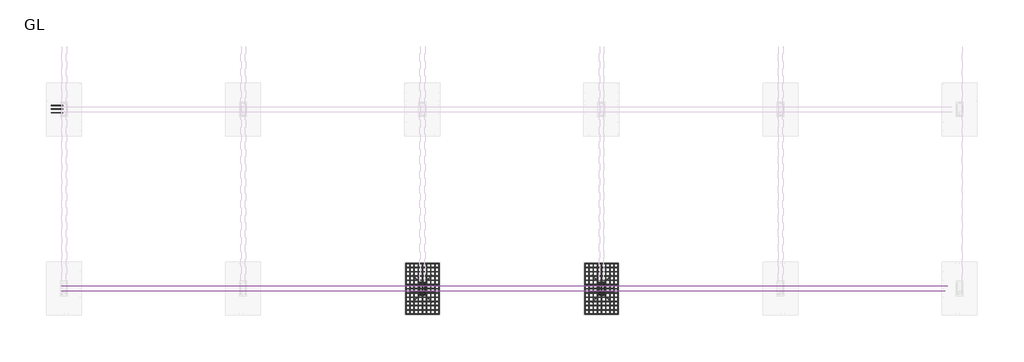
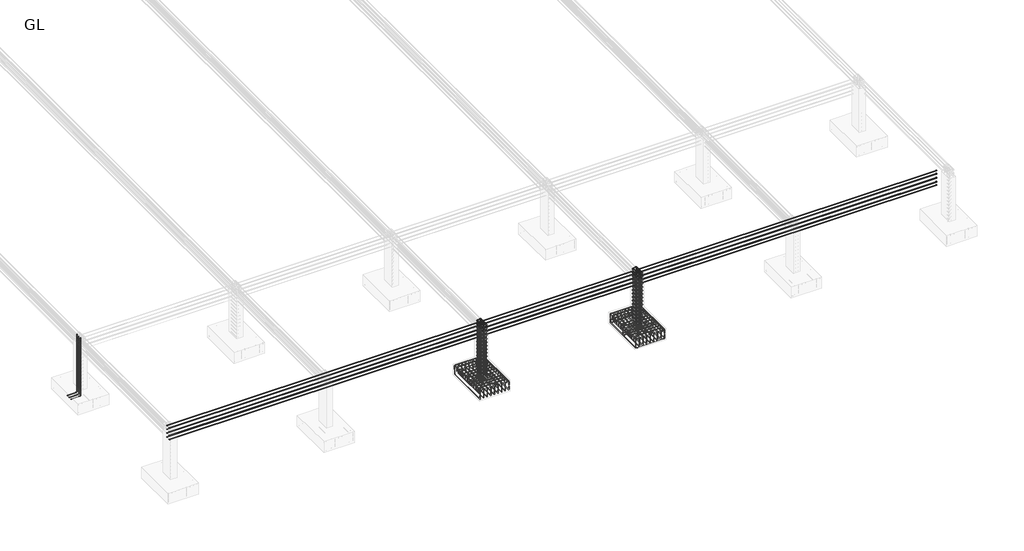
# One storey, part 3 of 16: 24 reinforcing bars.
"""IFC4 building model written with IfcOpenShell, lengths in millimetres."""

from ifc_helpers import new_model, si_unit, point, frame, origin, place, context, project, spatial, polyline, circle_curve, trimmed, segment, composite_curve, source, transform, mapped, element, save
from ifc_brep_helpers import swept_disk

model = new_model("IFC4")

# Units and contexts
model_context = context("Model", 3, world=origin())
ifc_project = project(units=[si_unit("LENGTHUNIT", "METRE", prefix="MILLI")], contexts=[model_context])

# Site, building, storey
site = spatial("IfcSite", under=ifc_project)
building = spatial("IfcBuilding", under=site)
storey = spatial("IfcBuildingStorey", under=building, Name="GL", Elevation=-1829.0)

# Reinforcing bars
placement = place(None, origin())
reinforcing_bar_shape = source(origin(), model_context, "Body", "SolidModel", [
    swept_disk(composite_curve([segment(polyline([(-11178.9544379, -19415.1167521, -2022.436678), (-11178.9544379, -19415.1167521, -1898.436678)]), True, "CONTINUOUS"), segment(trimmed(circle_curve(frame((-11148.9544379, -19415.1167521, -1898.436678), z_axis=(0.0, 1.0, 0.0), x_axis=(-30.0, 0.0, 0.0)), 30.0), [point((-11178.9544379, -19415.1167521, -1898.436678))], [point((-11148.9544379, -19415.1167521, -1868.436678))], True, "CARTESIAN"), True, "CONTINUOUS"), segment(polyline([(-11148.9544379, -19415.1167521, -1868.436678), (-10080.9544379, -19415.1167521, -1868.436678)]), True, "CONTINUOUS"), segment(trimmed(circle_curve(frame((-10080.9544379, -19415.1167521, -1898.436678), z_axis=(0.0, 1.0, 0.0), x_axis=(0.0, 0.0, 30.0)), 30.0), [point((-10080.9544379, -19415.1167521, -1868.436678))], [point((-10050.9544379, -19415.1167521, -1898.436678))], True, "CARTESIAN"), True, "CONTINUOUS"), segment(polyline([(-10050.9544379, -19415.1167521, -1898.436678), (-10050.9544379, -19415.1167521, -2022.436678)]), True, "CONTINUOUS")], self_intersect=False), 6.0),
])
element("IfcReinforcingBar", 1, at=placement, inside=storey, context=model_context, shape_type="MappedRepresentation", body=[
    mapped(reinforcing_bar_shape, transform((0.0, 0.0, 0.0), x_axis=(1.0, 0.0, 0.0), y_axis=(0.0, 1.0, 0.0), z_axis=(0.0, 0.0, 1.0))),
    mapped(reinforcing_bar_shape, transform((0.0, -144.0, 0.0), x_axis=(1.0, 0.0, 0.0), y_axis=(0.0, 1.0, 0.0), z_axis=(0.0, 0.0, 1.0))),
    mapped(reinforcing_bar_shape, transform((0.0, -288.0, 0.0), x_axis=(1.0, 0.0, 0.0), y_axis=(0.0, 1.0, 0.0), z_axis=(0.0, 0.0, 1.0))),
    mapped(reinforcing_bar_shape, transform((0.0, -432.0, 0.0), x_axis=(1.0, 0.0, 0.0), y_axis=(0.0, 1.0, 0.0), z_axis=(0.0, 0.0, 1.0))),
    mapped(reinforcing_bar_shape, transform((0.0, -576.0, 0.0), x_axis=(1.0, 0.0, 0.0), y_axis=(0.0, 1.0, 0.0), z_axis=(0.0, 0.0, 1.0))),
    mapped(reinforcing_bar_shape, transform((0.0, -720.0, 0.0), x_axis=(1.0, 0.0, 0.0), y_axis=(0.0, 1.0, 0.0), z_axis=(0.0, 0.0, 1.0))),
    mapped(reinforcing_bar_shape, transform((0.0, -864.0, 0.0), x_axis=(1.0, 0.0, 0.0), y_axis=(0.0, 1.0, 0.0), z_axis=(0.0, 0.0, 1.0))),
    mapped(reinforcing_bar_shape, transform((0.0, -1008.0, 0.0), x_axis=(1.0, 0.0, 0.0), y_axis=(0.0, 1.0, 0.0), z_axis=(0.0, 0.0, 1.0))),
    mapped(reinforcing_bar_shape, transform((0.0, -1152.0, 0.0), x_axis=(1.0, 0.0, 0.0), y_axis=(0.0, 1.0, 0.0), z_axis=(0.0, 0.0, 1.0))),
    mapped(reinforcing_bar_shape, transform((0.0, -1296.0, 0.0), x_axis=(1.0, 0.0, 0.0), y_axis=(0.0, 1.0, 0.0), z_axis=(0.0, 0.0, 1.0))),
    mapped(reinforcing_bar_shape, transform((0.0, -1440.0, 0.0), x_axis=(1.0, 0.0, 0.0), y_axis=(0.0, 1.0, 0.0), z_axis=(0.0, 0.0, 1.0))),
    mapped(reinforcing_bar_shape, transform((0.0, -1584.0, 0.0), x_axis=(1.0, 0.0, 0.0), y_axis=(0.0, 1.0, 0.0), z_axis=(0.0, 0.0, 1.0))),
    mapped(reinforcing_bar_shape, transform((0.0, -1728.0, 0.0), x_axis=(1.0, 0.0, 0.0), y_axis=(0.0, 1.0, 0.0), z_axis=(0.0, 0.0, 1.0))),
])
reinforcing_bar_2_shape = source(origin(), model_context, "Body", "SolidModel", [
    swept_disk(composite_curve([segment(polyline([(-11178.9544379, -21143.1167521, -2027.5081232), (-11178.9544379, -21143.1167521, -1903.5081232)]), True, "CONTINUOUS"), segment(trimmed(circle_curve(frame((-11178.9544379, -21113.1167521, -1903.5081232), z_axis=(-1.0, 0.0, 0.0), x_axis=(0.0, -30.0, 0.0)), 30.0), [point((-11178.9544379, -21143.1167521, -1903.5081232))], [point((-11178.9544379, -21113.1167521, -1873.5081232))], True, "CARTESIAN"), True, "CONTINUOUS"), segment(polyline([(-11178.9544379, -21113.1167521, -1873.5081232), (-11178.9544379, -19445.1167521, -1873.5081232)]), True, "CONTINUOUS"), segment(trimmed(circle_curve(frame((-11178.9544379, -19445.1167521, -1903.5081232), z_axis=(-1.0, 0.0, 0.0), x_axis=(0.0, 0.0, 30.0)), 30.0), [point((-11178.9544379, -19445.1167521, -1873.5081232))], [point((-11178.9544379, -19415.1167521, -1903.5081232))], True, "CARTESIAN"), True, "CONTINUOUS"), segment(polyline([(-11178.9544379, -19415.1167521, -1903.5081232), (-11178.9544379, -19415.1167521, -2027.5081232)]), True, "CONTINUOUS")], self_intersect=False), 6.0),
])
element("IfcReinforcingBar", 2, at=placement, inside=storey, context=model_context, shape_type="MappedRepresentation", body=[
    mapped(reinforcing_bar_2_shape, transform((0.0, 0.0, 0.0), x_axis=(1.0, 0.0, 0.0), y_axis=(0.0, 1.0, 0.0), z_axis=(0.0, 0.0, 1.0))),
    mapped(reinforcing_bar_2_shape, transform((141.0, 0.0, 0.0), x_axis=(1.0, 0.0, 0.0), y_axis=(0.0, 1.0, 0.0), z_axis=(0.0, 0.0, 1.0))),
    mapped(reinforcing_bar_2_shape, transform((282.0, 0.0, 0.0), x_axis=(1.0, 0.0, 0.0), y_axis=(0.0, 1.0, 0.0), z_axis=(0.0, 0.0, 1.0))),
    mapped(reinforcing_bar_2_shape, transform((423.0, 0.0, 0.0), x_axis=(1.0, 0.0, 0.0), y_axis=(0.0, 1.0, 0.0), z_axis=(0.0, 0.0, 1.0))),
    mapped(reinforcing_bar_2_shape, transform((564.0, 0.0, 0.0), x_axis=(1.0, 0.0, 0.0), y_axis=(0.0, 1.0, 0.0), z_axis=(0.0, 0.0, 1.0))),
    mapped(reinforcing_bar_2_shape, transform((705.0, 0.0, 0.0), x_axis=(1.0, 0.0, 0.0), y_axis=(0.0, 1.0, 0.0), z_axis=(0.0, 0.0, 1.0))),
    mapped(reinforcing_bar_2_shape, transform((846.0, 0.0, 0.0), x_axis=(1.0, 0.0, 0.0), y_axis=(0.0, 1.0, 0.0), z_axis=(0.0, 0.0, 1.0))),
    mapped(reinforcing_bar_2_shape, transform((987.0, 0.0, 0.0), x_axis=(1.0, 0.0, 0.0), y_axis=(0.0, 1.0, 0.0), z_axis=(0.0, 0.0, 1.0))),
    mapped(reinforcing_bar_2_shape, transform((1128.0, 0.0, 0.0), x_axis=(1.0, 0.0, 0.0), y_axis=(0.0, 1.0, 0.0), z_axis=(0.0, 0.0, 1.0))),
])
reinforcing_bar_3_shape = source(origin(), model_context, "Body", "SolidModel", [
    swept_disk(composite_curve([segment(polyline([(-10050.9544379, -21143.1167521, -2080.6239909), (-10050.9544379, -21143.1167521, -2204.6239909)]), True, "CONTINUOUS"), segment(trimmed(circle_curve(frame((-10050.9544379, -21113.1167521, -2204.6239909), z_axis=(1.0, 0.0, 0.0), x_axis=(0.0, -30.0, 0.0)), 30.0), [point((-10050.9544379, -21143.1167521, -2204.6239909))], [point((-10050.9544379, -21113.1167521, -2234.6239909))], True, "CARTESIAN"), True, "CONTINUOUS"), segment(polyline([(-10050.9544379, -21113.1167521, -2234.6239909), (-10050.9544379, -19458.1421892, -2234.6239909)]), True, "CONTINUOUS"), segment(trimmed(circle_curve(frame((-10050.9544379, -19458.1421892, -2204.6239909), z_axis=(1.0, 0.0, 0.0), x_axis=(0.0, 0.0, -30.0)), 30.0), [point((-10050.9544379, -19458.1421892, -2234.6239909))], [point((-10050.9544379, -19428.1421892, -2204.6239909))], True, "CARTESIAN"), True, "CONTINUOUS"), segment(polyline([(-10050.9544379, -19428.1421892, -2204.6239909), (-10050.9544379, -19428.1421892, -2080.6239909)]), True, "CONTINUOUS")], self_intersect=False), 6.0),
])
element("IfcReinforcingBar", 3, at=placement, inside=storey, context=model_context, shape_type="MappedRepresentation", body=[
    mapped(reinforcing_bar_3_shape, transform((0.0, 0.0, 0.0), x_axis=(1.0, 0.0, 0.0), y_axis=(0.0, 1.0, 0.0), z_axis=(0.0, 0.0, 1.0))),
    mapped(reinforcing_bar_3_shape, transform((-141.0, 0.0, 0.0), x_axis=(1.0, 0.0, 0.0), y_axis=(0.0, 1.0, 0.0), z_axis=(0.0, 0.0, 1.0))),
    mapped(reinforcing_bar_3_shape, transform((-282.0, 0.0, 0.0), x_axis=(1.0, 0.0, 0.0), y_axis=(0.0, 1.0, 0.0), z_axis=(0.0, 0.0, 1.0))),
    mapped(reinforcing_bar_3_shape, transform((-423.0, 0.0, 0.0), x_axis=(1.0, 0.0, 0.0), y_axis=(0.0, 1.0, 0.0), z_axis=(0.0, 0.0, 1.0))),
    mapped(reinforcing_bar_3_shape, transform((-564.0, 0.0, 0.0), x_axis=(1.0, 0.0, 0.0), y_axis=(0.0, 1.0, 0.0), z_axis=(0.0, 0.0, 1.0))),
    mapped(reinforcing_bar_3_shape, transform((-705.0, 0.0, 0.0), x_axis=(1.0, 0.0, 0.0), y_axis=(0.0, 1.0, 0.0), z_axis=(0.0, 0.0, 1.0))),
    mapped(reinforcing_bar_3_shape, transform((-846.0, 0.0, 0.0), x_axis=(1.0, 0.0, 0.0), y_axis=(0.0, 1.0, 0.0), z_axis=(0.0, 0.0, 1.0))),
    mapped(reinforcing_bar_3_shape, transform((-987.0, 0.0, 0.0), x_axis=(1.0, 0.0, 0.0), y_axis=(0.0, 1.0, 0.0), z_axis=(0.0, 0.0, 1.0))),
    mapped(reinforcing_bar_3_shape, transform((-1128.0, 0.0, 0.0), x_axis=(1.0, 0.0, 0.0), y_axis=(0.0, 1.0, 0.0), z_axis=(0.0, 0.0, 1.0))),
])
reinforcing_bar_4_shape = source(origin(), model_context, "Body", "SolidModel", [
    swept_disk(composite_curve([segment(polyline([(-3954.9544379, -19415.1167521, -2089.0), (-3954.9544379, -19415.1167521, -2213.0)]), True, "CONTINUOUS"), segment(trimmed(circle_curve(frame((-3984.9544379, -19415.1167521, -2213.0), z_axis=(0.0, 1.0, 0.0), x_axis=(30.0, 0.0, 0.0)), 30.0), [point((-3954.9544379, -19415.1167521, -2213.0))], [point((-3984.9544379, -19415.1167521, -2243.0))], True, "CARTESIAN"), True, "CONTINUOUS"), segment(polyline([(-3984.9544379, -19415.1167521, -2243.0), (-5052.9544379, -19415.1167521, -2243.0)]), True, "CONTINUOUS"), segment(trimmed(circle_curve(frame((-5052.9544379, -19415.1167521, -2213.0), z_axis=(0.0, 1.0, 0.0), x_axis=(0.0, 0.0, -30.0)), 30.0), [point((-5052.9544379, -19415.1167521, -2243.0))], [point((-5082.9544379, -19415.1167521, -2213.0))], True, "CARTESIAN"), True, "CONTINUOUS"), segment(polyline([(-5082.9544379, -19415.1167521, -2213.0), (-5082.9544379, -19415.1167521, -2089.0)]), True, "CONTINUOUS")], self_intersect=False), 6.0),
])
element("IfcReinforcingBar", 4, at=placement, inside=storey, context=model_context, shape_type="MappedRepresentation", body=[
    mapped(reinforcing_bar_4_shape, transform((0.0, 0.0, 0.0), x_axis=(1.0, 0.0, 0.0), y_axis=(0.0, 1.0, 0.0), z_axis=(0.0, 0.0, 1.0))),
    mapped(reinforcing_bar_4_shape, transform((0.0, -864.0, 0.0), x_axis=(1.0, 0.0, 0.0), y_axis=(0.0, 1.0, 0.0), z_axis=(0.0, 0.0, 1.0))),
    mapped(reinforcing_bar_4_shape, transform((0.0, -1728.0, 0.0), x_axis=(1.0, 0.0, 0.0), y_axis=(0.0, 1.0, 0.0), z_axis=(0.0, 0.0, 1.0))),
])
reinforcing_bar_5_shape = source(origin(), model_context, "Body", "SolidModel", [
    swept_disk(composite_curve([segment(polyline([(-5082.9544379, -19415.1167521, -2022.436678), (-5082.9544379, -19415.1167521, -1898.436678)]), True, "CONTINUOUS"), segment(trimmed(circle_curve(frame((-5052.9544379, -19415.1167521, -1898.436678), z_axis=(0.0, 1.0, 0.0), x_axis=(-30.0, 0.0, 0.0)), 30.0), [point((-5082.9544379, -19415.1167521, -1898.436678))], [point((-5052.9544379, -19415.1167521, -1868.436678))], True, "CARTESIAN"), True, "CONTINUOUS"), segment(polyline([(-5052.9544379, -19415.1167521, -1868.436678), (-3984.9544379, -19415.1167521, -1868.436678)]), True, "CONTINUOUS"), segment(trimmed(circle_curve(frame((-3984.9544379, -19415.1167521, -1898.436678), z_axis=(0.0, 1.0, 0.0), x_axis=(0.0, 0.0, 30.0)), 30.0), [point((-3984.9544379, -19415.1167521, -1868.436678))], [point((-3954.9544379, -19415.1167521, -1898.436678))], True, "CARTESIAN"), True, "CONTINUOUS"), segment(polyline([(-3954.9544379, -19415.1167521, -1898.436678), (-3954.9544379, -19415.1167521, -2022.436678)]), True, "CONTINUOUS")], self_intersect=False), 6.0),
])
element("IfcReinforcingBar", 5, at=placement, inside=storey, context=model_context, shape_type="MappedRepresentation", body=[
    mapped(reinforcing_bar_5_shape, transform((0.0, 0.0, 0.0), x_axis=(1.0, 0.0, 0.0), y_axis=(0.0, 1.0, 0.0), z_axis=(0.0, 0.0, 1.0))),
    mapped(reinforcing_bar_5_shape, transform((0.0, -144.0, 0.0), x_axis=(1.0, 0.0, 0.0), y_axis=(0.0, 1.0, 0.0), z_axis=(0.0, 0.0, 1.0))),
    mapped(reinforcing_bar_5_shape, transform((0.0, -288.0, 0.0), x_axis=(1.0, 0.0, 0.0), y_axis=(0.0, 1.0, 0.0), z_axis=(0.0, 0.0, 1.0))),
    mapped(reinforcing_bar_5_shape, transform((0.0, -432.0, 0.0), x_axis=(1.0, 0.0, 0.0), y_axis=(0.0, 1.0, 0.0), z_axis=(0.0, 0.0, 1.0))),
    mapped(reinforcing_bar_5_shape, transform((0.0, -576.0, 0.0), x_axis=(1.0, 0.0, 0.0), y_axis=(0.0, 1.0, 0.0), z_axis=(0.0, 0.0, 1.0))),
    mapped(reinforcing_bar_5_shape, transform((0.0, -720.0, 0.0), x_axis=(1.0, 0.0, 0.0), y_axis=(0.0, 1.0, 0.0), z_axis=(0.0, 0.0, 1.0))),
    mapped(reinforcing_bar_5_shape, transform((0.0, -864.0, 0.0), x_axis=(1.0, 0.0, 0.0), y_axis=(0.0, 1.0, 0.0), z_axis=(0.0, 0.0, 1.0))),
    mapped(reinforcing_bar_5_shape, transform((0.0, -1008.0, 0.0), x_axis=(1.0, 0.0, 0.0), y_axis=(0.0, 1.0, 0.0), z_axis=(0.0, 0.0, 1.0))),
    mapped(reinforcing_bar_5_shape, transform((0.0, -1152.0, 0.0), x_axis=(1.0, 0.0, 0.0), y_axis=(0.0, 1.0, 0.0), z_axis=(0.0, 0.0, 1.0))),
    mapped(reinforcing_bar_5_shape, transform((0.0, -1296.0, 0.0), x_axis=(1.0, 0.0, 0.0), y_axis=(0.0, 1.0, 0.0), z_axis=(0.0, 0.0, 1.0))),
    mapped(reinforcing_bar_5_shape, transform((0.0, -1440.0, 0.0), x_axis=(1.0, 0.0, 0.0), y_axis=(0.0, 1.0, 0.0), z_axis=(0.0, 0.0, 1.0))),
    mapped(reinforcing_bar_5_shape, transform((0.0, -1584.0, 0.0), x_axis=(1.0, 0.0, 0.0), y_axis=(0.0, 1.0, 0.0), z_axis=(0.0, 0.0, 1.0))),
    mapped(reinforcing_bar_5_shape, transform((0.0, -1728.0, 0.0), x_axis=(1.0, 0.0, 0.0), y_axis=(0.0, 1.0, 0.0), z_axis=(0.0, 0.0, 1.0))),
])
reinforcing_bar_6_shape = source(origin(), model_context, "Body", "SolidModel", [
    swept_disk(composite_curve([segment(polyline([(-5082.9544379, -21143.1167521, -2027.5081232), (-5082.9544379, -21143.1167521, -1903.5081232)]), True, "CONTINUOUS"), segment(trimmed(circle_curve(frame((-5082.9544379, -21113.1167521, -1903.5081232), z_axis=(-1.0, 0.0, 0.0), x_axis=(0.0, -30.0, 0.0)), 30.0), [point((-5082.9544379, -21143.1167521, -1903.5081232))], [point((-5082.9544379, -21113.1167521, -1873.5081232))], True, "CARTESIAN"), True, "CONTINUOUS"), segment(polyline([(-5082.9544379, -21113.1167521, -1873.5081232), (-5082.9544379, -19445.1167521, -1873.5081232)]), True, "CONTINUOUS"), segment(trimmed(circle_curve(frame((-5082.9544379, -19445.1167521, -1903.5081232), z_axis=(-1.0, 0.0, 0.0), x_axis=(0.0, 0.0, 30.0)), 30.0), [point((-5082.9544379, -19445.1167521, -1873.5081232))], [point((-5082.9544379, -19415.1167521, -1903.5081232))], True, "CARTESIAN"), True, "CONTINUOUS"), segment(polyline([(-5082.9544379, -19415.1167521, -1903.5081232), (-5082.9544379, -19415.1167521, -2027.5081232)]), True, "CONTINUOUS")], self_intersect=False), 6.0),
])
element("IfcReinforcingBar", 6, at=placement, inside=storey, context=model_context, shape_type="MappedRepresentation", body=[
    mapped(reinforcing_bar_6_shape, transform((0.0, 0.0, 0.0), x_axis=(1.0, 0.0, 0.0), y_axis=(0.0, 1.0, 0.0), z_axis=(0.0, 0.0, 1.0))),
    mapped(reinforcing_bar_6_shape, transform((141.0, 0.0, 0.0), x_axis=(1.0, 0.0, 0.0), y_axis=(0.0, 1.0, 0.0), z_axis=(0.0, 0.0, 1.0))),
    mapped(reinforcing_bar_6_shape, transform((282.0, 0.0, 0.0), x_axis=(1.0, 0.0, 0.0), y_axis=(0.0, 1.0, 0.0), z_axis=(0.0, 0.0, 1.0))),
    mapped(reinforcing_bar_6_shape, transform((423.0, 0.0, 0.0), x_axis=(1.0, 0.0, 0.0), y_axis=(0.0, 1.0, 0.0), z_axis=(0.0, 0.0, 1.0))),
    mapped(reinforcing_bar_6_shape, transform((564.0, 0.0, 0.0), x_axis=(1.0, 0.0, 0.0), y_axis=(0.0, 1.0, 0.0), z_axis=(0.0, 0.0, 1.0))),
    mapped(reinforcing_bar_6_shape, transform((705.0, 0.0, 0.0), x_axis=(1.0, 0.0, 0.0), y_axis=(0.0, 1.0, 0.0), z_axis=(0.0, 0.0, 1.0))),
    mapped(reinforcing_bar_6_shape, transform((846.0, 0.0, 0.0), x_axis=(1.0, 0.0, 0.0), y_axis=(0.0, 1.0, 0.0), z_axis=(0.0, 0.0, 1.0))),
    mapped(reinforcing_bar_6_shape, transform((987.0, 0.0, 0.0), x_axis=(1.0, 0.0, 0.0), y_axis=(0.0, 1.0, 0.0), z_axis=(0.0, 0.0, 1.0))),
    mapped(reinforcing_bar_6_shape, transform((1128.0, 0.0, 0.0), x_axis=(1.0, 0.0, 0.0), y_axis=(0.0, 1.0, 0.0), z_axis=(0.0, 0.0, 1.0))),
])
reinforcing_bar_7_shape = source(origin(), model_context, "Body", "SolidModel", [
    swept_disk(composite_curve([segment(polyline([(-3954.9544379, -21143.1167521, -2080.6239909), (-3954.9544379, -21143.1167521, -2204.6239909)]), True, "CONTINUOUS"), segment(trimmed(circle_curve(frame((-3954.9544379, -21113.1167521, -2204.6239909), z_axis=(1.0, 0.0, 0.0), x_axis=(0.0, -30.0, 0.0)), 30.0), [point((-3954.9544379, -21143.1167521, -2204.6239909))], [point((-3954.9544379, -21113.1167521, -2234.6239909))], True, "CARTESIAN"), True, "CONTINUOUS"), segment(polyline([(-3954.9544379, -21113.1167521, -2234.6239909), (-3954.9544379, -19458.1421892, -2234.6239909)]), True, "CONTINUOUS"), segment(trimmed(circle_curve(frame((-3954.9544379, -19458.1421892, -2204.6239909), z_axis=(1.0, 0.0, 0.0), x_axis=(0.0, 0.0, -30.0)), 30.0), [point((-3954.9544379, -19458.1421892, -2234.6239909))], [point((-3954.9544379, -19428.1421892, -2204.6239909))], True, "CARTESIAN"), True, "CONTINUOUS"), segment(polyline([(-3954.9544379, -19428.1421892, -2204.6239909), (-3954.9544379, -19428.1421892, -2080.6239909)]), True, "CONTINUOUS")], self_intersect=False), 6.0),
])
element("IfcReinforcingBar", 7, at=placement, inside=storey, context=model_context, shape_type="MappedRepresentation", body=[
    mapped(reinforcing_bar_7_shape, transform((0.0, 0.0, 0.0), x_axis=(1.0, 0.0, 0.0), y_axis=(0.0, 1.0, 0.0), z_axis=(0.0, 0.0, 1.0))),
    mapped(reinforcing_bar_7_shape, transform((-141.0, 0.0, 0.0), x_axis=(1.0, 0.0, 0.0), y_axis=(0.0, 1.0, 0.0), z_axis=(0.0, 0.0, 1.0))),
    mapped(reinforcing_bar_7_shape, transform((-282.0, 0.0, 0.0), x_axis=(1.0, 0.0, 0.0), y_axis=(0.0, 1.0, 0.0), z_axis=(0.0, 0.0, 1.0))),
    mapped(reinforcing_bar_7_shape, transform((-423.0, 0.0, 0.0), x_axis=(1.0, 0.0, 0.0), y_axis=(0.0, 1.0, 0.0), z_axis=(0.0, 0.0, 1.0))),
    mapped(reinforcing_bar_7_shape, transform((-564.0, 0.0, 0.0), x_axis=(1.0, 0.0, 0.0), y_axis=(0.0, 1.0, 0.0), z_axis=(0.0, 0.0, 1.0))),
    mapped(reinforcing_bar_7_shape, transform((-705.0, 0.0, 0.0), x_axis=(1.0, 0.0, 0.0), y_axis=(0.0, 1.0, 0.0), z_axis=(0.0, 0.0, 1.0))),
    mapped(reinforcing_bar_7_shape, transform((-846.0, 0.0, 0.0), x_axis=(1.0, 0.0, 0.0), y_axis=(0.0, 1.0, 0.0), z_axis=(0.0, 0.0, 1.0))),
    mapped(reinforcing_bar_7_shape, transform((-987.0, 0.0, 0.0), x_axis=(1.0, 0.0, 0.0), y_axis=(0.0, 1.0, 0.0), z_axis=(0.0, 0.0, 1.0))),
    mapped(reinforcing_bar_7_shape, transform((-1128.0, 0.0, 0.0), x_axis=(1.0, 0.0, 0.0), y_axis=(0.0, 1.0, 0.0), z_axis=(0.0, 0.0, 1.0))),
])
reinforcing_bar_8_shape = source(origin(), model_context, "Body", "SolidModel", [
    swept_disk(composite_curve([segment(polyline([(-22864.0642232, -14290.9117405, 241.0), (-22864.0642232, -14290.9117405, -2129.0)]), True, "CONTINUOUS"), segment(trimmed(circle_curve(frame((-22894.0642232, -14290.9117405, -2129.0), z_axis=(0.0, 1.0, 0.0), x_axis=(30.0, 0.0, 0.0)), 30.0), [point((-22864.0642232, -14290.9117405, -2129.0))], [point((-22894.0642232, -14290.9117405, -2159.0))], True, "CARTESIAN"), True, "CONTINUOUS"), segment(polyline([(-22894.0642232, -14290.9117405, -2159.0), (-23244.0642232, -14290.9117405, -2159.0)]), True, "CONTINUOUS")], self_intersect=False), 6.0),
])
element("IfcReinforcingBar", 8, at=placement, inside=storey, context=model_context, shape_type="MappedRepresentation", body=[
    mapped(reinforcing_bar_8_shape, transform((0.0, 0.0, 0.0), x_axis=(1.0, 0.0, 0.0), y_axis=(0.0, 1.0, 0.0), z_axis=(0.0, 0.0, 1.0))),
    mapped(reinforcing_bar_8_shape, transform((0.0, 123.5823926, 0.0), x_axis=(1.0, 0.0, 0.0), y_axis=(0.0, 1.0, 0.0), z_axis=(0.0, 0.0, 1.0))),
    mapped(reinforcing_bar_8_shape, transform((0.0, 247.1647853, 0.0), x_axis=(1.0, 0.0, 0.0), y_axis=(0.0, 1.0, 0.0), z_axis=(0.0, 0.0, 1.0))),
])
reinforcing_bar_9_shape = source(origin(), model_context, "Body", "SolidModel", [
    swept_disk(composite_curve([segment(polyline([(-10607.4864005, -20354.2223078, -1793.0), (-10695.1676414, -20441.9035486, -1793.0)]), True, "CONTINUOUS"), segment(trimmed(circle_curve(frame((-10673.9544379, -20463.1167521, -1793.0), z_axis=(0.0, 0.0, 1.0), x_axis=(-21.21320349999951, 21.21320349999951, 0.0)), 30.0), [point((-10695.1676414, -20441.9035486, -1793.0))], [point((-10673.9544379, -20493.1167521, -1793.0))], True, "CARTESIAN"), True, "CONTINUOUS"), segment(polyline([(-10673.9544379, -20493.1167521, -1793.0), (-10555.9544379, -20493.1167521, -1793.0)]), True, "CONTINUOUS"), segment(trimmed(circle_curve(frame((-10555.9544379, -20463.1167521, -1793.0), z_axis=(0.0, 0.0, 1.0), x_axis=(0.0, -30.0, 0.0)), 30.0), [point((-10555.9544379, -20493.1167521, -1793.0))], [point((-10525.9544379, -20463.1167521, -1793.0))], True, "CARTESIAN"), True, "CONTINUOUS"), segment(polyline([(-10525.9544379, -20463.1167521, -1793.0), (-10525.9544379, -20095.1167521, -1793.0)]), True, "CONTINUOUS"), segment(trimmed(circle_curve(frame((-10555.8864962, -20095.1167521, -1795.0178916), z_axis=(-0.06726305234213417, 0.0, 0.9977352764083365), x_axis=(29.93205830000079, 0.0, 2.0178915999999845)), 30.0), [point((-10525.9544379, -20095.1167521, -1793.0))], [point((-10555.8864962, -20065.1167521, -1795.0178916))], True, "CARTESIAN"), True, "CONTINUOUS"), segment(polyline([(-10555.8864962, -20065.1167521, -1795.0178916), (-10674.0223796, -20065.1167521, -1802.9821084)]), True, "CONTINUOUS"), segment(trimmed(circle_curve(frame((-10674.0223796, -20095.1167521, -1802.9821084), z_axis=(-0.06726305234213417, 0.0, 0.9977352764083365), x_axis=(0.0, 30.0, 0.0)), 30.0), [point((-10674.0223796, -20065.1167521, -1802.9821084))], [point((-10703.9544379, -20095.1167521, -1805.0))], True, "CARTESIAN"), True, "CONTINUOUS"), segment(polyline([(-10703.9544379, -20095.1167521, -1805.0), (-10703.9544379, -20463.1167521, -1805.0)]), True, "CONTINUOUS"), segment(trimmed(circle_curve(frame((-10673.9544379, -20463.1167521, -1805.0), z_axis=(0.0, 0.0, 1.0), x_axis=(-30.0, 0.0, 0.0)), 30.0), [point((-10703.9544379, -20463.1167521, -1805.0))], [point((-10652.7412345, -20484.3299555, -1805.0))], True, "CARTESIAN"), True, "CONTINUOUS"), segment(polyline([(-10652.7412345, -20484.3299555, -1805.0), (-10565.0599936, -20396.6487146, -1805.0)]), True, "CONTINUOUS")], self_intersect=False), 6.0),
])
element("IfcReinforcingBar", 9, at=placement, inside=storey, context=model_context, shape_type="MappedRepresentation", body=[
    mapped(reinforcing_bar_9_shape, transform((0.0, 0.0, 0.0), x_axis=(1.0, 0.0, 0.0), y_axis=(0.0, 1.0, 0.0), z_axis=(0.0, 0.0, 1.0))),
    mapped(reinforcing_bar_9_shape, transform((0.0, 0.0, 144.8571429), x_axis=(1.0, 0.0, 0.0), y_axis=(0.0, 1.0, 0.0), z_axis=(0.0, 0.0, 1.0))),
    mapped(reinforcing_bar_9_shape, transform((0.0, 0.0, 289.7142857), x_axis=(1.0, 0.0, 0.0), y_axis=(0.0, 1.0, 0.0), z_axis=(0.0, 0.0, 1.0))),
    mapped(reinforcing_bar_9_shape, transform((0.0, 0.0, 434.5714286), x_axis=(1.0, 0.0, 0.0), y_axis=(0.0, 1.0, 0.0), z_axis=(0.0, 0.0, 1.0))),
    mapped(reinforcing_bar_9_shape, transform((0.0, 0.0, 579.4285714), x_axis=(1.0, 0.0, 0.0), y_axis=(0.0, 1.0, 0.0), z_axis=(0.0, 0.0, 1.0))),
    mapped(reinforcing_bar_9_shape, transform((0.0, 0.0, 724.2857143), x_axis=(1.0, 0.0, 0.0), y_axis=(0.0, 1.0, 0.0), z_axis=(0.0, 0.0, 1.0))),
    mapped(reinforcing_bar_9_shape, transform((0.0, 0.0, 869.1428571), x_axis=(1.0, 0.0, 0.0), y_axis=(0.0, 1.0, 0.0), z_axis=(0.0, 0.0, 1.0))),
    mapped(reinforcing_bar_9_shape, transform((0.0, 0.0, 1014.0), x_axis=(1.0, 0.0, 0.0), y_axis=(0.0, 1.0, 0.0), z_axis=(0.0, 0.0, 1.0))),
    mapped(reinforcing_bar_9_shape, transform((0.0, 0.0, 1158.8571429), x_axis=(1.0, 0.0, 0.0), y_axis=(0.0, 1.0, 0.0), z_axis=(0.0, 0.0, 1.0))),
    mapped(reinforcing_bar_9_shape, transform((0.0, 0.0, 1303.7142857), x_axis=(1.0, 0.0, 0.0), y_axis=(0.0, 1.0, 0.0), z_axis=(0.0, 0.0, 1.0))),
    mapped(reinforcing_bar_9_shape, transform((0.0, 0.0, 1448.5714286), x_axis=(1.0, 0.0, 0.0), y_axis=(0.0, 1.0, 0.0), z_axis=(0.0, 0.0, 1.0))),
    mapped(reinforcing_bar_9_shape, transform((0.0, 0.0, 1593.4285714), x_axis=(1.0, 0.0, 0.0), y_axis=(0.0, 1.0, 0.0), z_axis=(0.0, 0.0, 1.0))),
    mapped(reinforcing_bar_9_shape, transform((0.0, 0.0, 1738.2857143), x_axis=(1.0, 0.0, 0.0), y_axis=(0.0, 1.0, 0.0), z_axis=(0.0, 0.0, 1.0))),
    mapped(reinforcing_bar_9_shape, transform((0.0, 0.0, 1883.1428571), x_axis=(1.0, 0.0, 0.0), y_axis=(0.0, 1.0, 0.0), z_axis=(0.0, 0.0, 1.0))),
    mapped(reinforcing_bar_9_shape, transform((0.0, 0.0, 2028.0), x_axis=(1.0, 0.0, 0.0), y_axis=(0.0, 1.0, 0.0), z_axis=(0.0, 0.0, 1.0))),
])
element("IfcReinforcingBar", 10, at=placement, inside=storey, context=model_context, shape_type="SolidModel", body=[
    swept_disk(composite_curve([segment(polyline([(-10672.0642232, -20464.0642439, 241.0), (-10672.0642232, -20464.0642439, -2129.0)]), True, "CONTINUOUS"), segment(trimmed(circle_curve(frame((-10693.2774266, -20485.2774473, -2129.0), z_axis=(-0.7071067811865187, 0.7071067811865764, 0.0), x_axis=(21.213203400000566, 21.213203399998747, 0.0)), 30.0), [point((-10672.0642232, -20464.0642439, -2129.0))], [point((-10693.2774266, -20485.2774473, -2159.0))], True, "CARTESIAN"), True, "CONTINUOUS"), segment(polyline([(-10693.2774266, -20485.2774473, -2159.0), (-10940.7648, -20732.7648207, -2159.0)]), True, "CONTINUOUS")], self_intersect=False), 6.0),
])
element("IfcReinforcingBar", 11, at=placement, inside=storey, context=model_context, shape_type="SolidModel", body=[
    swept_disk(composite_curve([segment(polyline([(-10672.0642232, -20094.1692603, 241.0), (-10672.0642232, -20094.1692603, -2129.0)]), True, "CONTINUOUS"), segment(trimmed(circle_curve(frame((-10693.2774266, -20072.9560568, -2129.0), z_axis=(0.7071067811865218, 0.7071067811865733, 0.0), x_axis=(21.213203400000566, -21.21320349999951, 0.0)), 30.0), [point((-10672.0642232, -20094.1692603, -2129.0))], [point((-10693.2774266, -20072.9560568, -2159.0))], True, "CARTESIAN"), True, "CONTINUOUS"), segment(polyline([(-10693.2774266, -20072.9560568, -2159.0), (-10940.7648, -19825.4686834, -2159.0)]), True, "CONTINUOUS")], self_intersect=False), 6.0),
])
element("IfcReinforcingBar", 12, at=placement, inside=storey, context=model_context, shape_type="SolidModel", body=[
    swept_disk(composite_curve([segment(polyline([(-10557.8446527, -20464.0642439, 241.0), (-10557.8446527, -20464.0642439, -2129.0)]), True, "CONTINUOUS"), segment(trimmed(circle_curve(frame((-10536.6314492, -20485.2774473, -2129.0), z_axis=(-0.7071067811865248, -0.7071067811865703, 0.0), x_axis=(-21.21320349999951, 21.213203399998747, 0.0)), 30.0), [point((-10557.8446527, -20464.0642439, -2129.0))], [point((-10536.6314492, -20485.2774473, -2159.0))], True, "CARTESIAN"), True, "CONTINUOUS"), segment(polyline([(-10536.6314492, -20485.2774473, -2159.0), (-10289.1440758, -20732.7648207, -2159.0)]), True, "CONTINUOUS")], self_intersect=False), 6.0),
])
element("IfcReinforcingBar", 13, at=placement, inside=storey, context=model_context, shape_type="SolidModel", body=[
    swept_disk(composite_curve([segment(polyline([(-10557.8446527, -20094.1692603, 241.0), (-10557.8446527, -20094.1692603, -2129.0)]), True, "CONTINUOUS"), segment(trimmed(circle_curve(frame((-10536.6314492, -20072.9560568, -2129.0), z_axis=(0.7071067811865157, -0.7071067811865794, 0.0), x_axis=(-21.21320349999951, -21.21320349999951, 0.0)), 30.0), [point((-10557.8446527, -20094.1692603, -2129.0))], [point((-10536.6314492, -20072.9560568, -2159.0))], True, "CARTESIAN"), True, "CONTINUOUS"), segment(polyline([(-10536.6314492, -20072.9560568, -2159.0), (-10289.1440758, -19825.4686834, -2159.0)]), True, "CONTINUOUS")], self_intersect=False), 6.0),
])
reinforcing_bar_10_shape = source(origin(), model_context, "Body", "SolidModel", [
    swept_disk(composite_curve([segment(polyline([(-10672.0642232, -20386.9117405, 241.0), (-10672.0642232, -20386.9117405, -2129.0)]), True, "CONTINUOUS"), segment(trimmed(circle_curve(frame((-10702.0642232, -20386.9117405, -2129.0), z_axis=(0.0, 1.0, 0.0), x_axis=(30.0, 0.0, 0.0)), 30.0), [point((-10672.0642232, -20386.9117405, -2129.0))], [point((-10702.0642232, -20386.9117405, -2159.0))], True, "CARTESIAN"), True, "CONTINUOUS"), segment(polyline([(-10702.0642232, -20386.9117405, -2159.0), (-11052.0642232, -20386.9117405, -2159.0)]), True, "CONTINUOUS")], self_intersect=False), 6.0),
])
element("IfcReinforcingBar", 14, at=placement, inside=storey, context=model_context, shape_type="MappedRepresentation", body=[
    mapped(reinforcing_bar_10_shape, transform((0.0, 0.0, 0.0), x_axis=(1.0, 0.0, 0.0), y_axis=(0.0, 1.0, 0.0), z_axis=(0.0, 0.0, 1.0))),
    mapped(reinforcing_bar_10_shape, transform((0.0, 123.5823926, 0.0), x_axis=(1.0, 0.0, 0.0), y_axis=(0.0, 1.0, 0.0), z_axis=(0.0, 0.0, 1.0))),
    mapped(reinforcing_bar_10_shape, transform((0.0, 247.1647853, 0.0), x_axis=(1.0, 0.0, 0.0), y_axis=(0.0, 1.0, 0.0), z_axis=(0.0, 0.0, 1.0))),
])
reinforcing_bar_11_shape = source(origin(), model_context, "Body", "SolidModel", [
    swept_disk(composite_curve([segment(polyline([(-10557.8446527, -20386.9117405, 241.0), (-10557.8446527, -20386.9117405, -2129.0)]), True, "CONTINUOUS"), segment(trimmed(circle_curve(frame((-10527.8446527, -20386.9117405, -2129.0), z_axis=(0.0, -1.0, 0.0), x_axis=(-30.0, 0.0, 0.0)), 30.0), [point((-10557.8446527, -20386.9117405, -2129.0))], [point((-10527.8446527, -20386.9117405, -2159.0))], True, "CARTESIAN"), True, "CONTINUOUS"), segment(polyline([(-10527.8446527, -20386.9117405, -2159.0), (-10177.8446527, -20386.9117405, -2159.0)]), True, "CONTINUOUS")], self_intersect=False), 6.0),
])
element("IfcReinforcingBar", 15, at=placement, inside=storey, context=model_context, shape_type="MappedRepresentation", body=[
    mapped(reinforcing_bar_11_shape, transform((0.0, 0.0, 0.0), x_axis=(1.0, 0.0, 0.0), y_axis=(0.0, 1.0, 0.0), z_axis=(0.0, 0.0, 1.0))),
    mapped(reinforcing_bar_11_shape, transform((0.0, 123.5823926, 0.0), x_axis=(1.0, 0.0, 0.0), y_axis=(0.0, 1.0, 0.0), z_axis=(0.0, 0.0, 1.0))),
    mapped(reinforcing_bar_11_shape, transform((0.0, 247.1647853, 0.0), x_axis=(1.0, 0.0, 0.0), y_axis=(0.0, 1.0, 0.0), z_axis=(0.0, 0.0, 1.0))),
])
reinforcing_bar_12_shape = source(origin(), model_context, "Body", "SolidModel", [
    swept_disk(composite_curve([segment(polyline([(-4511.4864005, -20354.2223078, -1793.0), (-4599.1676414, -20441.9035486, -1793.0)]), True, "CONTINUOUS"), segment(trimmed(circle_curve(frame((-4577.9544379, -20463.1167521, -1793.0), z_axis=(0.0, 0.0, 1.0), x_axis=(-21.213203500000418, 21.21320349999951, 0.0)), 30.0), [point((-4599.1676414, -20441.9035486, -1793.0))], [point((-4577.9544379, -20493.1167521, -1793.0))], True, "CARTESIAN"), True, "CONTINUOUS"), segment(polyline([(-4577.9544379, -20493.1167521, -1793.0), (-4459.9544379, -20493.1167521, -1793.0)]), True, "CONTINUOUS"), segment(trimmed(circle_curve(frame((-4459.9544379, -20463.1167521, -1793.0), z_axis=(0.0, 0.0, 1.0), x_axis=(0.0, -30.0, 0.0)), 30.0), [point((-4459.9544379, -20493.1167521, -1793.0))], [point((-4429.9544379, -20463.1167521, -1793.0))], True, "CARTESIAN"), True, "CONTINUOUS"), segment(polyline([(-4429.9544379, -20463.1167521, -1793.0), (-4429.9544379, -20095.1167521, -1793.0)]), True, "CONTINUOUS"), segment(trimmed(circle_curve(frame((-4459.8864962, -20095.1167521, -1795.0178916), z_axis=(-0.06726305234213417, 0.0, 0.9977352764083365), x_axis=(29.93205829999988, 0.0, 2.0178915999999845)), 30.0), [point((-4429.9544379, -20095.1167521, -1793.0))], [point((-4459.8864962, -20065.1167521, -1795.0178916))], True, "CARTESIAN"), True, "CONTINUOUS"), segment(polyline([(-4459.8864962, -20065.1167521, -1795.0178916), (-4578.0223796, -20065.1167521, -1802.9821084)]), True, "CONTINUOUS"), segment(trimmed(circle_curve(frame((-4578.0223796, -20095.1167521, -1802.9821084), z_axis=(-0.06726305234213417, 0.0, 0.9977352764083365), x_axis=(0.0, 30.0, 0.0)), 30.0), [point((-4578.0223796, -20065.1167521, -1802.9821084))], [point((-4607.9544379, -20095.1167521, -1805.0))], True, "CARTESIAN"), True, "CONTINUOUS"), segment(polyline([(-4607.9544379, -20095.1167521, -1805.0), (-4607.9544379, -20463.1167521, -1805.0)]), True, "CONTINUOUS"), segment(trimmed(circle_curve(frame((-4577.9544379, -20463.1167521, -1805.0), z_axis=(0.0, 0.0, 1.0), x_axis=(-30.0, 0.0, 0.0)), 30.0), [point((-4607.9544379, -20463.1167521, -1805.0))], [point((-4556.7412345, -20484.3299555, -1805.0))], True, "CARTESIAN"), True, "CONTINUOUS"), segment(polyline([(-4556.7412345, -20484.3299555, -1805.0), (-4469.0599936, -20396.6487146, -1805.0)]), True, "CONTINUOUS")], self_intersect=False), 6.0),
])
element("IfcReinforcingBar", 16, at=placement, inside=storey, context=model_context, shape_type="MappedRepresentation", body=[
    mapped(reinforcing_bar_12_shape, transform((0.0, 0.0, 0.0), x_axis=(1.0, 0.0, 0.0), y_axis=(0.0, 1.0, 0.0), z_axis=(0.0, 0.0, 1.0))),
    mapped(reinforcing_bar_12_shape, transform((0.0, 0.0, 144.8571429), x_axis=(1.0, 0.0, 0.0), y_axis=(0.0, 1.0, 0.0), z_axis=(0.0, 0.0, 1.0))),
    mapped(reinforcing_bar_12_shape, transform((0.0, 0.0, 289.7142857), x_axis=(1.0, 0.0, 0.0), y_axis=(0.0, 1.0, 0.0), z_axis=(0.0, 0.0, 1.0))),
    mapped(reinforcing_bar_12_shape, transform((0.0, 0.0, 434.5714286), x_axis=(1.0, 0.0, 0.0), y_axis=(0.0, 1.0, 0.0), z_axis=(0.0, 0.0, 1.0))),
    mapped(reinforcing_bar_12_shape, transform((0.0, 0.0, 579.4285714), x_axis=(1.0, 0.0, 0.0), y_axis=(0.0, 1.0, 0.0), z_axis=(0.0, 0.0, 1.0))),
    mapped(reinforcing_bar_12_shape, transform((0.0, 0.0, 724.2857143), x_axis=(1.0, 0.0, 0.0), y_axis=(0.0, 1.0, 0.0), z_axis=(0.0, 0.0, 1.0))),
    mapped(reinforcing_bar_12_shape, transform((0.0, 0.0, 869.1428571), x_axis=(1.0, 0.0, 0.0), y_axis=(0.0, 1.0, 0.0), z_axis=(0.0, 0.0, 1.0))),
    mapped(reinforcing_bar_12_shape, transform((0.0, 0.0, 1014.0), x_axis=(1.0, 0.0, 0.0), y_axis=(0.0, 1.0, 0.0), z_axis=(0.0, 0.0, 1.0))),
    mapped(reinforcing_bar_12_shape, transform((0.0, 0.0, 1158.8571429), x_axis=(1.0, 0.0, 0.0), y_axis=(0.0, 1.0, 0.0), z_axis=(0.0, 0.0, 1.0))),
    mapped(reinforcing_bar_12_shape, transform((0.0, 0.0, 1303.7142857), x_axis=(1.0, 0.0, 0.0), y_axis=(0.0, 1.0, 0.0), z_axis=(0.0, 0.0, 1.0))),
    mapped(reinforcing_bar_12_shape, transform((0.0, 0.0, 1448.5714286), x_axis=(1.0, 0.0, 0.0), y_axis=(0.0, 1.0, 0.0), z_axis=(0.0, 0.0, 1.0))),
    mapped(reinforcing_bar_12_shape, transform((0.0, 0.0, 1593.4285714), x_axis=(1.0, 0.0, 0.0), y_axis=(0.0, 1.0, 0.0), z_axis=(0.0, 0.0, 1.0))),
    mapped(reinforcing_bar_12_shape, transform((0.0, 0.0, 1738.2857143), x_axis=(1.0, 0.0, 0.0), y_axis=(0.0, 1.0, 0.0), z_axis=(0.0, 0.0, 1.0))),
    mapped(reinforcing_bar_12_shape, transform((0.0, 0.0, 1883.1428571), x_axis=(1.0, 0.0, 0.0), y_axis=(0.0, 1.0, 0.0), z_axis=(0.0, 0.0, 1.0))),
    mapped(reinforcing_bar_12_shape, transform((0.0, 0.0, 2028.0), x_axis=(1.0, 0.0, 0.0), y_axis=(0.0, 1.0, 0.0), z_axis=(0.0, 0.0, 1.0))),
])
element("IfcReinforcingBar", 17, at=placement, inside=storey, context=model_context, shape_type="SolidModel", body=[
    swept_disk(composite_curve([segment(polyline([(-4576.0642232, -20464.0642439, 241.0), (-4576.0642232, -20464.0642439, -2129.0)]), True, "CONTINUOUS"), segment(trimmed(circle_curve(frame((-4597.2774266, -20485.2774473, -2129.0), z_axis=(-0.7071067811865187, 0.7071067811865764, 0.0), x_axis=(21.213203399999657, 21.213203399998747, 0.0)), 30.0), [point((-4576.0642232, -20464.0642439, -2129.0))], [point((-4597.2774266, -20485.2774473, -2159.0))], True, "CARTESIAN"), True, "CONTINUOUS"), segment(polyline([(-4597.2774266, -20485.2774473, -2159.0), (-4844.7648, -20732.7648207, -2159.0)]), True, "CONTINUOUS")], self_intersect=False), 6.0),
])
element("IfcReinforcingBar", 18, at=placement, inside=storey, context=model_context, shape_type="SolidModel", body=[
    swept_disk(composite_curve([segment(polyline([(-4576.0642232, -20094.1692603, 241.0), (-4576.0642232, -20094.1692603, -2129.0)]), True, "CONTINUOUS"), segment(trimmed(circle_curve(frame((-4597.2774266, -20072.9560568, -2129.0), z_axis=(0.7071067811865218, 0.7071067811865733, 0.0), x_axis=(21.213203399999657, -21.21320349999951, 0.0)), 30.0), [point((-4576.0642232, -20094.1692603, -2129.0))], [point((-4597.2774266, -20072.9560568, -2159.0))], True, "CARTESIAN"), True, "CONTINUOUS"), segment(polyline([(-4597.2774266, -20072.9560568, -2159.0), (-4844.7648, -19825.4686834, -2159.0)]), True, "CONTINUOUS")], self_intersect=False), 6.0),
])
element("IfcReinforcingBar", 19, at=placement, inside=storey, context=model_context, shape_type="SolidModel", body=[
    swept_disk(composite_curve([segment(polyline([(-4461.8446527, -20464.0642439, 241.0), (-4461.8446527, -20464.0642439, -2129.0)]), True, "CONTINUOUS"), segment(trimmed(circle_curve(frame((-4440.6314492, -20485.2774473, -2129.0), z_axis=(-0.7071067811865248, -0.7071067811865703, 0.0), x_axis=(-21.21320349999951, 21.213203399998747, 0.0)), 30.0), [point((-4461.8446527, -20464.0642439, -2129.0))], [point((-4440.6314492, -20485.2774473, -2159.0))], True, "CARTESIAN"), True, "CONTINUOUS"), segment(polyline([(-4440.6314492, -20485.2774473, -2159.0), (-4193.1440758, -20732.7648207, -2159.0)]), True, "CONTINUOUS")], self_intersect=False), 6.0),
])
element("IfcReinforcingBar", 20, at=placement, inside=storey, context=model_context, shape_type="SolidModel", body=[
    swept_disk(composite_curve([segment(polyline([(-4461.8446527, -20094.1692603, 241.0), (-4461.8446527, -20094.1692603, -2129.0)]), True, "CONTINUOUS"), segment(trimmed(circle_curve(frame((-4440.6314492, -20072.9560568, -2129.0), z_axis=(0.7071067811865157, -0.7071067811865794, 0.0), x_axis=(-21.21320349999951, -21.21320349999951, 0.0)), 30.0), [point((-4461.8446527, -20094.1692603, -2129.0))], [point((-4440.6314492, -20072.9560568, -2159.0))], True, "CARTESIAN"), True, "CONTINUOUS"), segment(polyline([(-4440.6314492, -20072.9560568, -2159.0), (-4193.1440758, -19825.4686834, -2159.0)]), True, "CONTINUOUS")], self_intersect=False), 6.0),
])
reinforcing_bar_13_shape = source(origin(), model_context, "Body", "SolidModel", [
    swept_disk(composite_curve([segment(polyline([(-4576.0642232, -20386.9117405, 241.0), (-4576.0642232, -20386.9117405, -2129.0)]), True, "CONTINUOUS"), segment(trimmed(circle_curve(frame((-4606.0642232, -20386.9117405, -2129.0), z_axis=(0.0, 1.0, 0.0), x_axis=(30.0, 0.0, 0.0)), 30.0), [point((-4576.0642232, -20386.9117405, -2129.0))], [point((-4606.0642232, -20386.9117405, -2159.0))], True, "CARTESIAN"), True, "CONTINUOUS"), segment(polyline([(-4606.0642232, -20386.9117405, -2159.0), (-4956.0642232, -20386.9117405, -2159.0)]), True, "CONTINUOUS")], self_intersect=False), 6.0),
])
element("IfcReinforcingBar", 21, at=placement, inside=storey, context=model_context, shape_type="MappedRepresentation", body=[
    mapped(reinforcing_bar_13_shape, transform((0.0, 0.0, 0.0), x_axis=(1.0, 0.0, 0.0), y_axis=(0.0, 1.0, 0.0), z_axis=(0.0, 0.0, 1.0))),
    mapped(reinforcing_bar_13_shape, transform((0.0, 123.5823926, 0.0), x_axis=(1.0, 0.0, 0.0), y_axis=(0.0, 1.0, 0.0), z_axis=(0.0, 0.0, 1.0))),
    mapped(reinforcing_bar_13_shape, transform((0.0, 247.1647853, 0.0), x_axis=(1.0, 0.0, 0.0), y_axis=(0.0, 1.0, 0.0), z_axis=(0.0, 0.0, 1.0))),
])
reinforcing_bar_14_shape = source(origin(), model_context, "Body", "SolidModel", [
    swept_disk(composite_curve([segment(polyline([(-4461.8446527, -20386.9117405, 241.0), (-4461.8446527, -20386.9117405, -2129.0)]), True, "CONTINUOUS"), segment(trimmed(circle_curve(frame((-4431.8446527, -20386.9117405, -2129.0), z_axis=(0.0, -1.0, 0.0), x_axis=(-30.0, 0.0, 0.0)), 30.0), [point((-4461.8446527, -20386.9117405, -2129.0))], [point((-4431.8446527, -20386.9117405, -2159.0))], True, "CARTESIAN"), True, "CONTINUOUS"), segment(polyline([(-4431.8446527, -20386.9117405, -2159.0), (-4081.8446527, -20386.9117405, -2159.0)]), True, "CONTINUOUS")], self_intersect=False), 6.0),
])
element("IfcReinforcingBar", 22, at=placement, inside=storey, context=model_context, shape_type="MappedRepresentation", body=[
    mapped(reinforcing_bar_14_shape, transform((0.0, 0.0, 0.0), x_axis=(1.0, 0.0, 0.0), y_axis=(0.0, 1.0, 0.0), z_axis=(0.0, 0.0, 1.0))),
    mapped(reinforcing_bar_14_shape, transform((0.0, 123.5823926, 0.0), x_axis=(1.0, 0.0, 0.0), y_axis=(0.0, 1.0, 0.0), z_axis=(0.0, 0.0, 1.0))),
    mapped(reinforcing_bar_14_shape, transform((0.0, 247.1647853, 0.0), x_axis=(1.0, 0.0, 0.0), y_axis=(0.0, 1.0, 0.0), z_axis=(0.0, 0.0, 1.0))),
])
reinforcing_bar_15_shape = source(origin(), model_context, "Body", "SolidModel", [
    swept_disk(composite_curve([segment(polyline([(7246.2567543, -20187.7503796, 211.9770044), (-22901.9544379, -20187.7503796, 211.9770044)]), True, "CONTINUOUS")], self_intersect=False), 6.0),
])
element("IfcReinforcingBar", 23, at=placement, inside=storey, context=model_context, shape_type="MappedRepresentation", body=[
    mapped(reinforcing_bar_15_shape, transform((0.0, 0.0, 0.0), x_axis=(1.0, 0.0, 0.0), y_axis=(0.0, 1.0, 0.0), z_axis=(0.0, 0.0, 1.0))),
    mapped(reinforcing_bar_15_shape, transform((0.0, 0.0, -160.0851188), x_axis=(1.0, 0.0, 0.0), y_axis=(0.0, 1.0, 0.0), z_axis=(0.0, 0.0, 1.0))),
    mapped(reinforcing_bar_15_shape, transform((0.0, 0.0, -320.1702376), x_axis=(1.0, 0.0, 0.0), y_axis=(0.0, 1.0, 0.0), z_axis=(0.0, 0.0, 1.0))),
    mapped(reinforcing_bar_15_shape, transform((0.0, 0.0, -480.2553564), x_axis=(1.0, 0.0, 0.0), y_axis=(0.0, 1.0, 0.0), z_axis=(0.0, 0.0, 1.0))),
])
reinforcing_bar_16_shape = source(origin(), model_context, "Body", "SolidModel", [
    swept_disk(composite_curve([segment(polyline([(7153.4199035, -20355.3263285, -262.6869429), (-22901.9544379, -20355.3263285, -262.6869429)]), True, "CONTINUOUS")], self_intersect=False), 6.0),
])
element("IfcReinforcingBar", 24, at=placement, inside=storey, context=model_context, shape_type="MappedRepresentation", body=[
    mapped(reinforcing_bar_16_shape, transform((0.0, 0.0, 0.0), x_axis=(1.0, 0.0, 0.0), y_axis=(0.0, 1.0, 0.0), z_axis=(0.0, 0.0, 1.0))),
    mapped(reinforcing_bar_16_shape, transform((0.0, 0.0, 158.2213158), x_axis=(1.0, 0.0, 0.0), y_axis=(0.0, 1.0, 0.0), z_axis=(0.0, 0.0, 1.0))),
    mapped(reinforcing_bar_16_shape, transform((0.0, 0.0, 316.4426315), x_axis=(1.0, 0.0, 0.0), y_axis=(0.0, 1.0, 0.0), z_axis=(0.0, 0.0, 1.0))),
    mapped(reinforcing_bar_16_shape, transform((0.0, 0.0, 474.6639473), x_axis=(1.0, 0.0, 0.0), y_axis=(0.0, 1.0, 0.0), z_axis=(0.0, 0.0, 1.0))),
])

save(model, "model.ifc")

# Revit data of these elements
# Elements 1, 2, 3, 4, 5, 6, 7, 8, 9, 10, 11, 12, 13, 14, 15, 16, 17, 18, 19, 20, 21, 22, 23, 24 (IfcReinforcingBar)
#   Phase Created = New Construction
